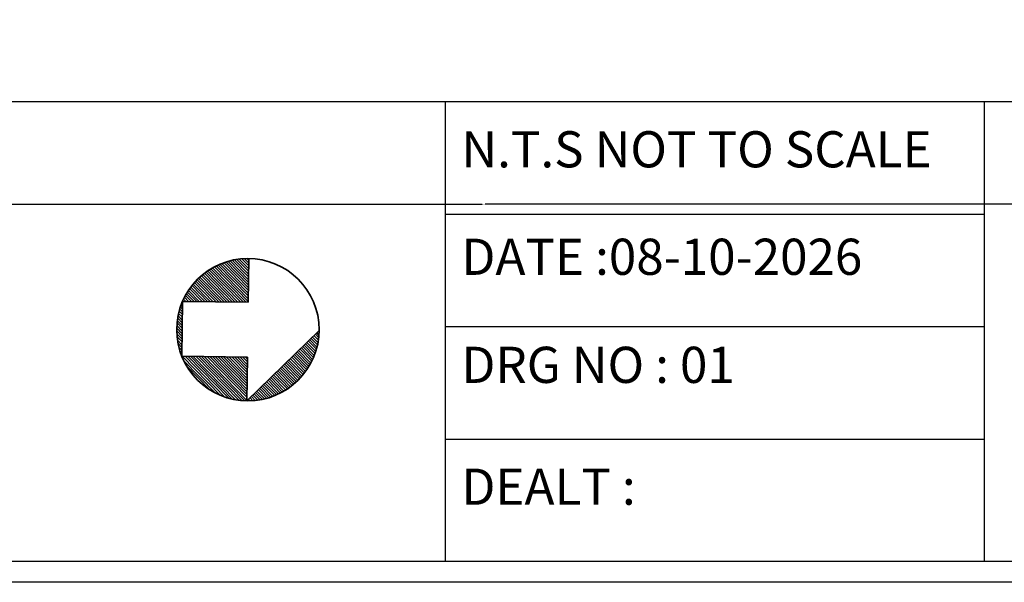
# Model space of a CAD drawing. Units: inches. Extents: x 84 to 1044, y -280 to 906.
# Tile 2 of 105: x 441 to 700, y -280 to -132. Entities that reach past the tile are written whole.
import ezdxf

# ---------------------------------------------------------------- set-up
doc = ezdxf.new("R2010")
doc.units = ezdxf.units.IN
for name, color, linetype, lineweight in [('A-ANNO-DIMS', 2, 'Continuous', 18), ('A-ANNO-SYMB', 7, 'Continuous', 15), ('A-ANNO-TTLB', 7, 'Continuous', 25), ('walls', 250, 'Continuous', 35)]:
    doc.layers.add(name, color=color, linetype=linetype, lineweight=lineweight)
doc.styles.add('1-100DIM', font='txt', dxfattribs={"height": 0.3})
doc.styles.get("Standard").update_dxf_attribs({"font": 'arial.ttf'})
doc.dimstyles.get("Standard").update_dxf_attribs({"dimtxt": 0.18, "dimasz": 0.18, "dimexe": 0.18, "dimexo": 0.0625, "dimgap": 0.09, "dimtad": 0, "dimtih": 1, "dimtoh": 1, "dimdec": 4, "dimzin": 0, "dimdsep": 46, "dimtxsty": 'Standard', "dimcen": 0.09, "dimadec": 0, "dimazin": 0, "dimtfac": 1, "dimtdec": 4, "dimtofl": 0, "dimtmove": 0, "dimatfit": 3, "dimfxl": 1, "dimtolj": 1, "dimtzin": 0, "dimarcsym": 0})

# ---------------------------------------------------------------- blocks, each defined once
blk = doc.blocks.new('NORTH')
at = {"layer": 'walls'}
h = blk.add_hatch(dxfattribs=at)
h.set_pattern_fill('ANSI31', color=256, scale=6.087211)
h.set_pattern_definition([(45, (-41048.0969, 128612.4242), (-0.53803848, 0.53803848), [])])
h.paths.add_polyline_path([(6704.42, -25696.22), (6687.22, -25696.22, 0.302843), (6704.42, -25722.01)])
h.paths.add_polyline_path([(6743.1, -25696.22), (6725.9, -25696.22), (6725.9, -25722.01, 0.302843)])
h.paths.add_polyline_path([(6715.16, -25668.28), (6743.1, -25696.22, 0.414214)])
h.paths.add_polyline_path([(6725.9, -25722.01), (6704.42, -25722.01, 0.199872)])
for p, q in [((6743.1, -25696.22, 0.29), (6715.16, -25668.28, 0.29)), ((6687.22, -25696.22, 0.29), (6704.42, -25696.22, 0.29)), ((6704.42, -25722.01, 0.29), (6704.42, -25696.22, 0.29)), ((6725.9, -25722.01, 0.29), (6725.9, -25696.22, 0.29)), ((6725.9, -25696.22, 0.29), (6743.1, -25696.22, 0.29)), ((6704.42, -25722.01, 0.29), (6725.9, -25722.01, 0.29))]:
    blk.add_line(p, q, dxfattribs=at)
blk.add_circle((6715.16, -25696.22, 0.29), 27.94, dxfattribs=at)
blk = doc.blocks.new('*D60')
at = {"layer": 'A-ANNO-DIMS', "color": 0, "lineweight": -2, "transparency": 16777216}
for p, q in [((134.18, -121.94), (134.18, -180.64)), ((992.07, -121.94), (992.07, -180.64)), ((134.36, -180.46), (562.73, -180.46)), ((991.89, -180.46), (563.52, -180.46))]:
    blk.add_line(p, q, dxfattribs=at)
at = {"layer": 'A-ANNO-DIMS', "color": 0, "transparency": 16777216}
for points in [[(134.36, -180.43), (134.36, -180.49), (134.18, -180.46)], [(991.89, -180.43), (991.89, -180.49), (992.07, -180.46)]]:
    blk.add_solid(points, dxfattribs=at)
at = {"layer": 'Defpoints', "color": 0, "transparency": 16777216}
for p in [(134.18, -121.88), (992.07, -121.88), (992.07, -180.46)]:
    blk.add_point(p, dxfattribs=at)
at = {"layer": 'A-ANNO-DIMS', "color": 0, "transparency": 16777216, "insert": (563.13, -180.46), "char_height": 0.18, "attachment_point": 5}
blk.add_mtext('\\A1;857.9', dxfattribs=at)

msp = doc.modelspace()

# ---------------------------------------------------------------- linework, layer by layer
at = {"layer": 'A-ANNO-TTLB'}
for p, q in [((106.576, -153.519), (1021.832, -153.519)), ((553.155, -274.288), (553.155, -153.519)), ((694.537, -153.519), (694.537, -274.288)), ((553.155, -183.055), (694.537, -183.055)), ((553.155, -212.591), (694.537, -212.591)), ((553.155, -242.126), (694.537, -242.126))]:
    msp.add_line(p, q, dxfattribs=at)
for points in [[(101.1, 905.916), (1027.308, 905.916), (1027.308, -279.764), (101.1, -279.764)], [(106.576, 900.439), (1021.832, 900.439), (1021.832, -274.288), (106.576, -274.288)]]:
    msp.add_lwpolyline(points, close=True, dxfattribs=at)

# ---------------------------------------------------------------- block references
at = {"layer": 'A-ANNO-SYMB', "xscale": 0.6693256603733035, "yscale": 0.6693256603733035, "zscale": 0.6693256603733035, "rotation": 269.2509902977627}
msp.add_blockref('NORTH', (17757.663, 4055.999, -0.196), dxfattribs=at)

# ---------------------------------------------------------------- texts
at = {"layer": 'A-ANNO-TTLB', "char_height": 9.50132, "attachment_point": 1, "style": '1-100DIM'}
for s, insert in [('{\\f@Malgun Gothic|b0|i0|c0|p34;N.T.S NOT TO SCALE }', (557.316, -161.289)), ('{\\f@Malgun Gothic|b0|i0|c0|p34;DATE :08-10-2026}', (557.316, -189.512)), ('{\\f@Malgun Gothic|b0|i0|c0|p34;DRG NO : 01}', (557.316, -217.897)), ('{\\f@Malgun Gothic|b0|i0|c0|p34;DEALT :}', (557.316, -249.897))]:
    msp.add_mtext_dynamic_manual_height_columns(s, width=268.28376, gutter_width=14.846, heights=[0], dxfattribs=dict(at, insert=insert))

# ---------------------------------------------------------------- dimensions: what is measured, and where the dimension line sits
at = {"layer": 'A-ANNO-DIMS'}
dim = msp.add_linear_dim(base=(992.074, -180.46), p1=(134.179, -121.88), p2=(992.074, -121.88), dimstyle='Standard', override={"dimdec": 1, "dimlfac": 1, "dimrnd": 0, "dimzin": 0, "dimdsep": 46, "dimlunit": 2}, dxfattribs=at)
dim.commit()
dim.dimension.update_dxf_attribs({"geometry": '*D60', "text_midpoint": (563.127, -180.46)})

doc.saveas('drawing.dxf')
